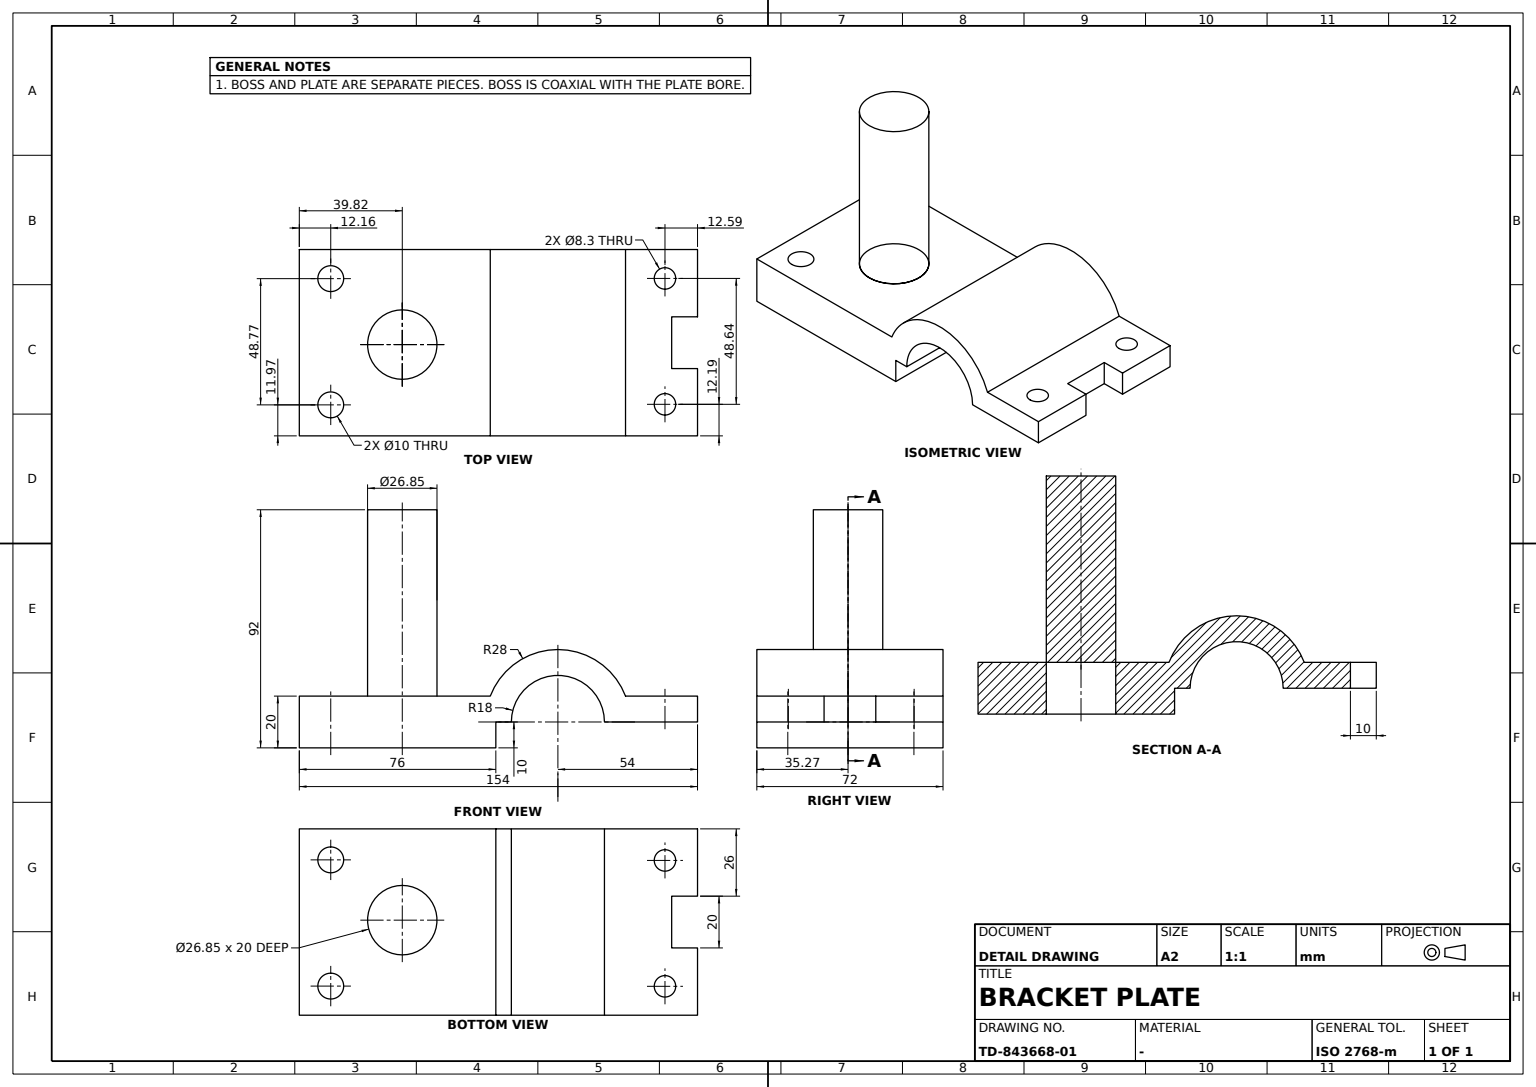
CATIA V5 part; units mm, degrees
sketch "Sketch1" plane through (0, 0, 0) normal (1, 0, 0) x (0, 1, 0)
  line L0 (77, 10) -> (77, 0)
  line L1 (-1, -10) -> (-77, -10)
  line L2 (-77, -10) -> (-77, 10)
  line L3 (-77, 10) -> (-3.1534, 10)
  point P0 (77, 10)
  point P1 (77, -10)
  point P2 (-77, -10)
  arc A0 (41, 0) -> (5, 0) centre (23, 0) ccw
  point P3 (23, 0)
  arc A1 (49.1534, 10) -> (-3.1534, 10) centre (23, 0) ccw
  line L4 (77, 0) -> (41, 0)
  point P4 (77, 0)
  point P5 (23, 0)
  line L5 (5, 0) -> (-1, 0)
  point P6 (5, 0)
  line L6 (-1, 0) -> (-1, -10)
  line L7 (49.1534, 10) -> (77, 10)
  point P7 (49.1534, 10)
  point P8 (49.1534, 10)
  dimension "radius A1" = 28
  dimension "radius A0" = 18
  dimension "length L6" = 10
  dimension "distance P1 P2" = 154
  dimension "distance P0 P1" = 20
  dimension "distance P4 P5" = 54
  constraint vertical L0 y-axis
  constraint vertical L2 y-axis
  constraint vertical L6 y-axis
  constraint horizontal L1 x-axis
  constraint horizontal L3 x-axis
  constraint horizontal L4 x-axis
  constraint horizontal L5 x-axis
  constraint horizontal L7 x-axis
  constraint equidistance L0 L2 origin
  constraint equidistance L1 L3 origin
  constraint coincidence P5 P3
  constraint coincidence P6 L4
  constraint coincidence A1 P7
  constraint coincidence L3 L7
  constraint coincidence L7 P8
  constraint coincidence P7 P8
extrude "Pad1" add sketch "Sketch1" against normal blind 72
sketch "Sketch2" plane through (0, 0, 10) normal (0, 0, 1) x (1, 0, 0)
  point P0 (-36, 72)
  line L0 (-26, 77) -> (-26, 67)
  line L1 (-26, 67) -> (-46, 67)
  line L2 (-46, 67) -> (-46, 77)
  line L3 (-46, 77) -> (-26, 77)
  line L4 (0, 77) -> (-72, 77) construction
  line L5 (-72, 77) -> (-72, 49.1534) construction
  dimension "length L3" = 20
  dimension "length L0" = 10
  dimension "distance P0 L5" = 36
  constraint vertical L0 y-axis
  constraint vertical L2 y-axis
  constraint horizontal L1 x-axis
  constraint horizontal L3 x-axis
  constraint equidistance L0 L2 P0
  constraint equidistance L1 L3 P0
  constraint coincidence L3 L4
extrude "Pocket1" cut sketch "Sketch2" against normal blind 72
sketch "Sketch3" plane through (0, 0, 10) normal (0, 0, 1) x (1, 0, 0)
  circle A0 centre (-35.2694, -37.1801) radius 13.4228
  circle A1 centre (-60.7477, -64.8423) radius 5
  circle A2 centre (-11.9749, -64.8423) radius 5
  dimension "radius A1" = 5
  dimension "radius A2" = 5
extrude "Pad2" add sketch "Sketch3" along normal blind 72 contours A0
extrude "Pocket2" cut sketch "Sketch3" against normal blind 72
sketch "Sketch4" plane through (0, 0, 10) normal (0, 0, 1) x (1, 0, 0)
  circle A0 centre (-60.8342, 64.4109) radius 4.1499
  circle A1 centre (-12.1919, 64.4109) radius 4.1499
  dimension "radius A1" = 4.1499
  dimension "radius A0" = 4.1499
extrude "Pocket3" cut sketch "Sketch4" against normal blind 72
